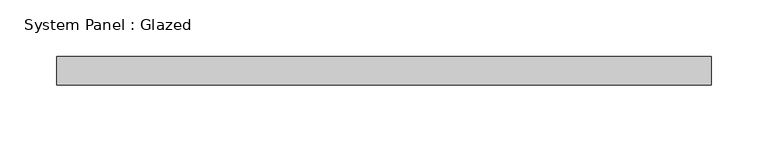
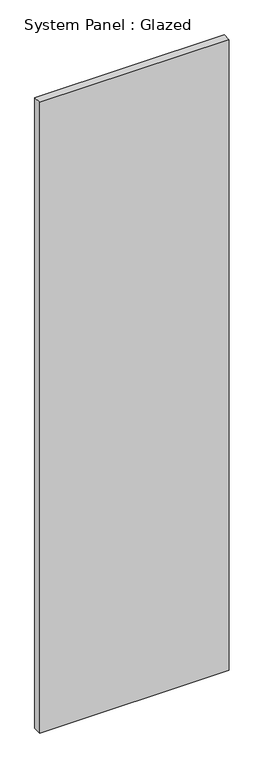
"""IFC4 building model written with IfcOpenShell, lengths in millimetres: plate geometry, System Panel : Glazed."""

from ifc_helpers import new_model, si_unit, origin, origin_with_axes, place, context, project, spatial, polyline, outline, extrude, source, transform, mapped, element, save


def system_panel_glazed_b4fc352e(model_context):
    return source(origin(), model_context, "Body", "SweptSolid", [
        extrude(outline(polyline([(288.925, 19.05), (-288.925, 19.05), (-288.925, 44.45), (288.925, 44.45), (288.925, 19.05)])), origin_with_axes(), (0.0, 0.0, 1.0), 2032.0),
    ])


if __name__ == "__main__":
    model = new_model("IFC4")
    model_context = context("Model", 3, world=origin())
    ifc_project = project(units=[si_unit("LENGTHUNIT", "METRE", prefix="MILLI")], contexts=[model_context])
    site = spatial("IfcSite", under=ifc_project)
    building = spatial("IfcBuilding", under=site)
    placement = place(None, origin())
    system_panel_glazed_shape = system_panel_glazed_b4fc352e(model_context)
    element("IfcPlate", 1, ObjectType="System Panel : Glazed", at=placement, inside=building, context=model_context, shape_type="MappedRepresentation", body=[
        mapped(system_panel_glazed_shape, transform((0.0, 0.0, 0.0), x_axis=(1.0, 0.0, 0.0), y_axis=(0.0, 1.0, 0.0), z_axis=(0.0, 0.0, 1.0))),
    ])
    save(model, "model.ifc")

# Revit data of these elements
# Type "System Panel : Glazed"
#   Construction Type Id = "GSP4R"
#   Analytic Construction = "1/8 in Pilkington single glazing"
#   Visual Light Transmittance = 0.9
#   Solar Heat Gain Coefficient = 0.86
#   Heat Transfer Coefficient (U) = 1.18115 BTU/(h·ft²·°F)
#   Define Thermal Properties by = 1
# Element 1 (IfcPlate, "System Panel : Glazed")
#   Materials on its faces: "Glass"
# Materials
#   "Glass": class "Glass", colour RGB 0 128 192, transparency 0.75, Description = "Soda Lime Glass", Cost = 0
